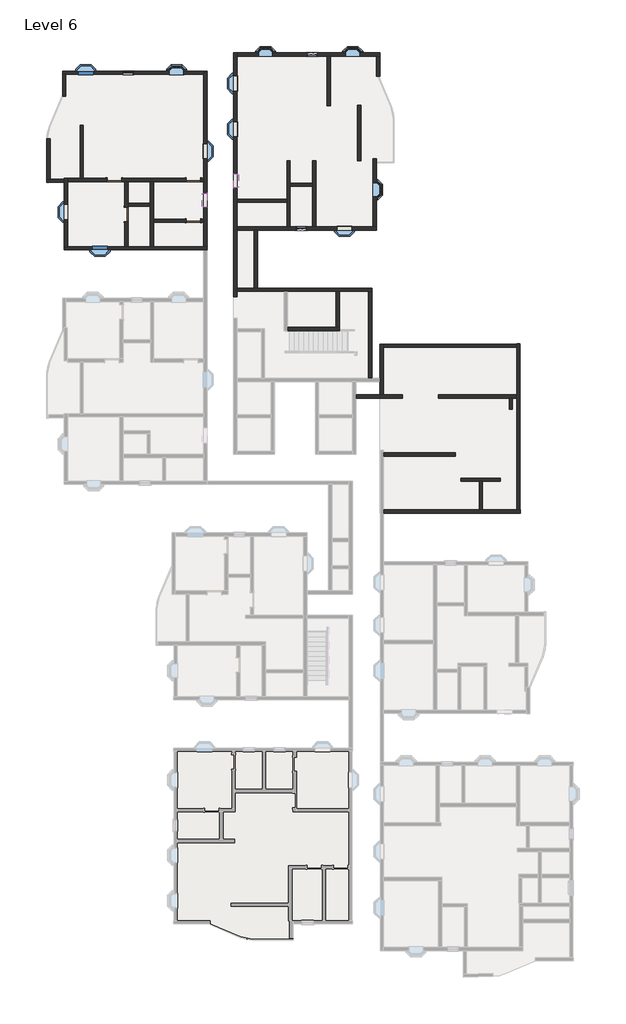
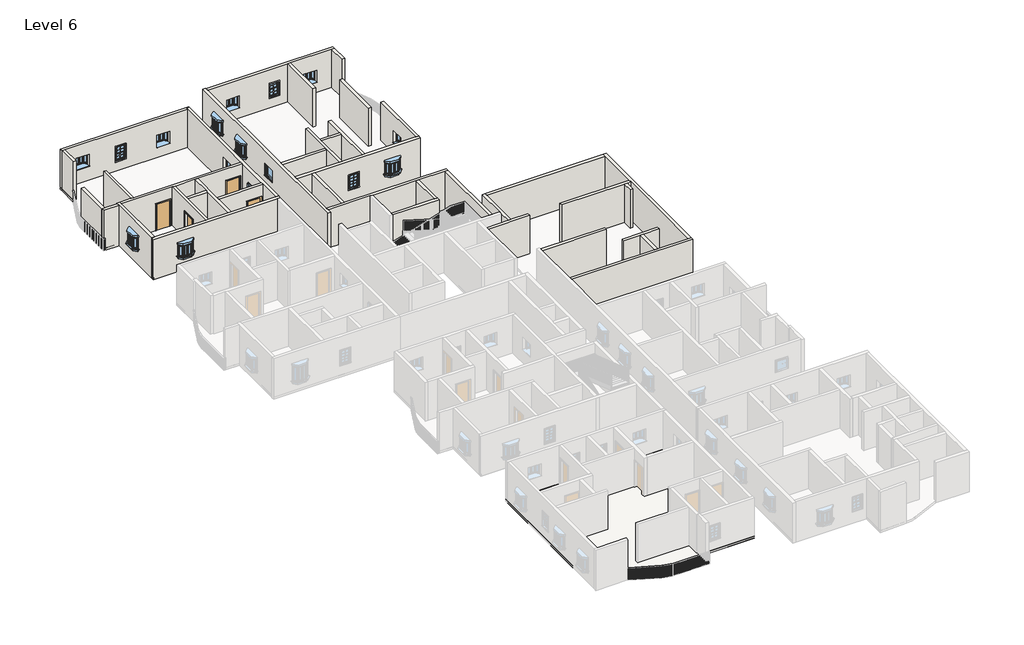
# One storey, part 4 of 14: 39 walls, 16 windows, 4 doors, 2 roofs.
"""IFC4 building model written with IfcOpenShell, lengths in millimetres."""

from ifc_helpers import new_model, si_unit, point, frame, frame_2d, origin, place, context, project, spatial, polyline, circle_curve, trimmed, segment, composite_curve, outline, extrude, faceted_brep, transform, mapped, element, save
from components import door_719f80de, window_910x910mm_67ef725a, window_8debb0fa, windows_sgl_w_glazing_bars_910x910mm_256712d0

model = new_model("IFC4")

# Units and contexts
model_context = context("Model", 3, world=origin())
ifc_project = project(units=[si_unit("LENGTHUNIT", "METRE", prefix="MILLI")], contexts=[model_context])

# Site, building, storey
site = spatial("IfcSite", under=ifc_project)
building = spatial("IfcBuilding", under=site)
storey = spatial("IfcBuildingStorey", under=building, Name="Level 6", Elevation=15240.0)

# Doors
placement = place(None, origin())
door_shape = door_719f80de(model_context)
element("IfcDoor", 1, ObjectType="Single-Flush : 36\" x 84\"", at=placement, inside=storey, context=model_context, shape_type="MappedRepresentation", body=[
    mapped(door_shape, transform((-16068.1391351, 22048.4083494, 15240.0), x_axis=(1.0, 0.0, 0.0), y_axis=(0.0, 1.0, 0.0), z_axis=(0.0, 0.0, 1.0))),
])
element("IfcDoor", 2, ObjectType="Single-Flush : 36\" x 84\"", at=placement, inside=storey, context=model_context, shape_type="MappedRepresentation", body=[
    mapped(door_shape, transform((-15306.1391351, 19864.0083494, 15240.0), x_axis=(0.0, 1.0, 0.0), y_axis=(-1.0, 0.0, 0.0), z_axis=(0.0, 0.0, 1.0))),
])
element("IfcDoor", 3, ObjectType="Single-Flush : 36\" x 84\"", at=placement, inside=storey, context=model_context, shape_type="MappedRepresentation", body=[
    mapped(door_shape, transform((-11057.9891351, 19470.3083494, 15240.0), x_axis=(1.0, 0.0, 0.0), y_axis=(0.0, 1.0, 0.0), z_axis=(0.0, 0.0, 1.0))),
])
element("IfcDoor", 4, ObjectType="Single-Flush : 36\" x 84\"", at=placement, inside=storey, context=model_context, shape_type="MappedRepresentation", body=[
    mapped(door_shape, transform((-11057.9891351, 22048.4083494, 15240.0), x_axis=(1.0, 0.0, 0.0), y_axis=(0.0, 1.0, 0.0), z_axis=(0.0, 0.0, 1.0))),
])

# Roofs
element("IfcRoof", 5, ObjectType="Generic - 12\"", at=placement, inside=storey, context=model_context, shape_type="SweptSolid", body=[
    extrude(outline(composite_curve([segment(polyline([(-10024.8708389, -25100.3416506), (-12290.487215, -25100.3416506), (-12290.487215, -13962.4416506), (-986.8891351, -13962.4416506), (-986.8891351, -25100.3416506), (-4746.0891351, -25100.3416506), (-4746.0891351, -26090.9416506), (-7315.6413127, -26090.9416506)]), True, "CONTINUOUS"), segment(trimmed(circle_curve(frame_2d((-7315.6413127, -24160.5416506)), 1930.4), [point((-7315.6413127, -26090.9416506))], [point((-8075.5356374, -25935.0851906))], False, "CARTESIAN"), True, "CONTINUOUS"), segment(polyline([(-8075.5356374, -25935.0851906), (-10024.8708389, -25100.3416506)]), True, "CONTINUOUS")], self_intersect=False)), frame((0.0, 0.0, 15240.0), z_axis=(0.0, 0.0, 1.0), x_axis=(1.0, 0.0, 0.0)), (0.0, 0.0, 1.0), 152.4),
])
element("IfcRoof", 6, ObjectType="Generic - 12\"", at=placement, inside=storey, context=model_context, shape_type="SweptSolid", body=[
    extrude(outline(composite_curve([segment(polyline([(-10024.8708389, -25100.3416506), (-12290.487215, -25100.3416506), (-12290.487215, -13962.4416506), (-986.8891351, -13962.4416506), (-986.8891351, -25100.3416506), (-4746.0891351, -25100.3416506), (-4746.0891351, -26090.9416506), (-7315.6413127, -26090.9416506)]), True, "CONTINUOUS"), segment(trimmed(circle_curve(frame_2d((-7315.6413127, -24160.5416506)), 1930.4), [point((-7315.6413127, -26090.9416506))], [point((-8075.5356374, -25935.0851906))], False, "CARTESIAN"), True, "CONTINUOUS"), segment(polyline([(-8075.5356374, -25935.0851906), (-10024.8708389, -25100.3416506)]), True, "CONTINUOUS")], self_intersect=False)), frame((0.0, 0.0, 15240.0), z_axis=(0.0, 0.0, 1.0), x_axis=(1.0, 0.0, 0.0)), (0.0, 0.0, 1.0), 152.4),
])

# Walls
element("IfcWall", 7, ObjectType="4.5\" p", at=placement, inside=storey, context=model_context, shape_type="Brep", body=[
    faceted_brep([(-10600.7891351, 21946.8083494, 17373.6), (-10600.7891351, 21946.8083494, 15240.0), (-10397.5891351, 21946.8083494, 15240.0), (-10397.5891351, 21946.8083494, 18288.0), (-13578.9391351, 21946.8083494, 18288.0), (-13782.1391351, 21946.8083494, 18288.0), (-15204.5391351, 21946.8083494, 18288.0), (-15407.7391351, 21946.8083494, 18288.0), (-19033.5891351, 21946.8083494, 18288.0), (-19033.5891351, 21946.8083494, 15240.0), (-16525.3391351, 21946.8083494, 15240.0), (-16525.3391351, 21946.8083494, 17373.6), (-15610.9391351, 21946.8083494, 17373.6), (-15610.9391351, 21946.8083494, 15240.0), (-15407.7391351, 21946.8083494, 15240.0), (-15204.5391351, 21946.8083494, 15240.0), (-13782.1391351, 21946.8083494, 15240.0), (-13578.9391351, 21946.8083494, 15240.0), (-11515.1891351, 21946.8083494, 15240.0), (-11515.1891351, 21946.8083494, 17373.6), (-10397.5891351, 22150.0083494, 15240.0), (-10600.7891351, 22150.0083494, 15240.0), (-10600.7891351, 22150.0083494, 17373.6), (-11515.1891351, 22150.0083494, 17373.6), (-11515.1891351, 22150.0083494, 15240.0), (-15610.9391351, 22150.0083494, 15240.0), (-15610.9391351, 22150.0083494, 17373.6), (-16525.3391351, 22150.0083494, 17373.6), (-16525.3391351, 22150.0083494, 15240.0), (-18042.9891351, 22150.0083494, 15240.0), (-18246.1891351, 22150.0083494, 15240.0), (-19033.5891351, 22150.0083494, 15240.0), (-19033.5891351, 22150.0083494, 18288.0), (-18246.1891351, 22150.0083494, 18288.0), (-18042.9891351, 22150.0083494, 18288.0), (-10397.5891351, 22150.0083494, 18288.0)], [[[0, 1, 2, 3, 4, 5, 6, 7, 8, 9, 10, 11, 12, 13, 14, 15, 16, 17, 18, 19]], [[20, 21, 22, 23, 24, 25, 26, 27, 28, 29, 30, 31, 32, 33, 34, 35]], [[10, 9, 31, 30, 29, 28]], [[2, 1, 21, 20]], [[18, 17, 16, 15, 14, 13, 25, 24]], [[8, 7, 6, 5, 4, 3, 35, 34, 33, 32]], [[9, 8, 32, 31]], [[3, 2, 20, 35]], [[26, 25, 13, 12]], [[27, 26, 12, 11]], [[28, 27, 11, 10]], [[22, 21, 1, 0]], [[23, 22, 0, 19]], [[24, 23, 19, 18]]]),
])
element("IfcWall", 8, ObjectType="4.5\" p", at=placement, inside=storey, context=model_context, shape_type="Brep", body=[
    faceted_brep([(-15407.7391351, 21946.8083494, 15240.0), (-15407.7391351, 20321.2083494, 15240.0), (-15407.7391351, 20321.2083494, 17373.6), (-15407.7391351, 19406.8083494, 17373.6), (-15407.7391351, 19406.8083494, 15240.0), (-15407.7391351, 17812.9583494, 15240.0), (-15407.7391351, 17812.9583494, 18288.0), (-15407.7391351, 21946.8083494, 18288.0), (-15204.5391351, 20321.2083494, 17373.6), (-15204.5391351, 20321.2083494, 15240.0), (-15204.5391351, 20372.0083494, 15240.0), (-15204.5391351, 20575.2083494, 15240.0), (-15204.5391351, 21946.8083494, 15240.0), (-15204.5391351, 21946.8083494, 18288.0), (-15204.5391351, 20575.2083494, 18288.0), (-15204.5391351, 20372.0083494, 18288.0), (-15204.5391351, 17812.9583494, 18288.0), (-15204.5391351, 17812.9583494, 15240.0), (-15204.5391351, 19406.8083494, 15240.0), (-15204.5391351, 19406.8083494, 17373.6)], [[[0, 1, 2, 3, 4, 5, 6, 7]], [[8, 9, 10, 11, 12, 13, 14, 15, 16, 17, 18, 19]], [[18, 17, 5, 4]], [[12, 11, 10, 9, 1, 0]], [[7, 6, 16, 15, 14, 13]], [[6, 5, 17, 16]], [[0, 7, 13, 12]], [[2, 1, 9, 8]], [[3, 2, 8, 19]], [[4, 3, 19, 18]]]),
])
element("IfcWall", 9, ObjectType="4.5\" p", at=placement, inside=storey, context=model_context, shape_type="Brep", body=[
    faceted_brep([(-13782.1391351, 21946.8083494, 15240.0), (-13782.1391351, 20575.2083494, 15240.0), (-13782.1391351, 20372.0083494, 15240.0), (-13782.1391351, 17812.9583494, 15240.0), (-13782.1391351, 17812.9583494, 18288.0), (-13782.1391351, 20372.0083494, 18288.0), (-13782.1391351, 20575.2083494, 18288.0), (-13782.1391351, 21946.8083494, 18288.0), (-13578.9391351, 21946.8083494, 15240.0), (-13578.9391351, 21946.8083494, 18288.0), (-13578.9391351, 19571.9083494, 18288.0), (-13578.9391351, 19368.7083494, 18288.0), (-13578.9391351, 17812.9583494, 18288.0), (-13578.9391351, 17812.9583494, 15240.0), (-13578.9391351, 19368.7083494, 15240.0), (-13578.9391351, 19571.9083494, 15240.0)], [[[0, 1, 2, 3, 4, 5, 6, 7]], [[8, 9, 10, 11, 12, 13, 14, 15]], [[3, 2, 1, 0, 8, 15, 14, 13]], [[7, 6, 5, 4, 12, 11, 10, 9]], [[4, 3, 13, 12]], [[0, 7, 9, 8]]]),
])
element("IfcWall", 10, ObjectType="4.5\" p", at=placement, inside=storey, context=model_context, shape_type="SweptSolid", body=[
    extrude(outline(polyline([(-13782.1391351, 20372.0083494), (-15204.5391351, 20372.0083494), (-15204.5391351, 20575.2083494), (-13782.1391351, 20575.2083494), (-13782.1391351, 20372.0083494)])), frame((0.0, 0.0, 15240.0), z_axis=(0.0, 0.0, 1.0), x_axis=(1.0, 0.0, 0.0)), (0.0, 0.0, 1.0), 3048.0),
])
element("IfcWall", 11, ObjectType="4.5\" p", at=placement, inside=storey, context=model_context, shape_type="SweptSolid", body=[
    extrude(outline(polyline([(17373.6, -10600.7891351), (15240.0, -10600.7891351), (15240.0, -10397.5891351), (18288.0, -10397.5891351), (18288.0, -13578.9391351), (15240.0, -13578.9391351), (15240.0, -11515.1891351), (17373.6, -11515.1891351), (17373.6, -10600.7891351)])), frame((0.0, 19368.7083494, 0.0), z_axis=(0.0, 1.0, 0.0), x_axis=(0.0, 0.0, 1.0)), (0.0, 0.0, 1.0), 203.2),
])
element("IfcWall", 12, ObjectType="4.5\" p", at=placement, inside=storey, context=model_context, shape_type="SweptSolid", body=[
    extrude(outline(polyline([(-18246.1891351, 22150.0083494), (-18246.1891351, 25515.5083494), (-18042.9891351, 25515.5083494), (-18042.9891351, 22150.0083494), (-18246.1891351, 22150.0083494)])), frame((0.0, 0.0, 15240.0), z_axis=(0.0, 0.0, 1.0), x_axis=(1.0, 0.0, 0.0)), (0.0, 0.0, 1.0), 3048.0),
])
element("IfcWall", 13, ObjectType="4.5\" p", at=placement, inside=storey, context=model_context, shape_type="SweptSolid", body=[
    extrude(outline(polyline([(-6993.9891351, 18875.1215905), (-6993.9891351, 15192.1215905), (-7197.1891351, 15192.1215905), (-7197.1891351, 18875.1215905), (-6993.9891351, 18875.1215905)])), frame((0.0, 0.0, 15240.0), z_axis=(0.0, 0.0, 1.0), x_axis=(1.0, 0.0, 0.0)), (0.0, 0.0, 1.0), 3048.0),
])
element("IfcWall", 14, ObjectType="4.5\" p", at=placement, inside=storey, context=model_context, shape_type="Brep", body=[
    faceted_brep([(-8289.3891351, 18875.1215905, 15240.0), (-7197.1891351, 18875.1215905, 15240.0), (-6993.9891351, 18875.1215905, 15240.0), (562.5108649, 18875.1215905, 15240.0), (562.5108649, 18875.1215905, 18288.0), (-6993.9891351, 18875.1215905, 18288.0), (-7197.1891351, 18875.1215905, 18288.0), (-8289.3891351, 18875.1215905, 18288.0), (-1017.6641351, 18875.1215905, 17350.0), (-1017.6641351, 18875.1215905, 16440.0), (-1927.6641351, 18875.1215905, 16440.0), (-1927.6641351, 18875.1215905, 17350.0), (-3876.1391351, 18875.1215905, 17221.2), (-3876.1391351, 18875.1215905, 16154.4), (-4536.5391351, 18875.1215905, 16154.4), (-4536.5391351, 18875.1215905, 17221.2), (-8289.3891351, 19078.3215905, 15240.0), (-8289.3891351, 19078.3215905, 18288.0), (-5120.7391351, 19078.3215905, 18288.0), (-4917.5391351, 19078.3215905, 18288.0), (-3495.1391351, 19078.3215905, 18288.0), (-3291.9391351, 19078.3215905, 18288.0), (346.6108649, 19078.3215905, 18288.0), (549.8108649, 19078.3215905, 18288.0), (562.5108649, 19078.3215905, 18288.0), (562.5108649, 19078.3215905, 15240.0), (549.8108649, 19078.3215905, 15240.0), (346.6108649, 19078.3215905, 15240.0), (-3291.9391351, 19078.3215905, 15240.0), (-3495.1391351, 19078.3215905, 15240.0), (-4917.5391351, 19078.3215905, 15240.0), (-5120.7391351, 19078.3215905, 15240.0), (-1017.6641351, 19078.3215905, 17350.0), (-1927.6641351, 19078.3215905, 17350.0), (-1927.6641351, 19078.3215905, 16440.0), (-1017.6641351, 19078.3215905, 16440.0), (-3876.1391351, 19078.3215905, 17221.2), (-4536.5391351, 19078.3215905, 17221.2), (-4536.5391351, 19078.3215905, 16154.4), (-3876.1391351, 19078.3215905, 16154.4)], [[[0, 1, 2, 3, 4, 5, 6, 7], [8, 9, 10, 11], [12, 13, 14, 15]], [[16, 17, 18, 19, 20, 21, 22, 23, 24, 25, 26, 27, 28, 29, 30, 31], [32, 33, 34, 35], [36, 37, 38, 39]], [[3, 2, 1, 0, 16, 31, 30, 29, 28, 27, 26, 25]], [[4, 3, 25, 24]], [[7, 6, 5, 4, 24, 23, 22, 21, 20, 19, 18, 17]], [[0, 7, 17, 16]], [[9, 8, 32, 35]], [[10, 9, 35, 34]], [[11, 10, 34, 33]], [[8, 11, 33, 32]], [[13, 12, 36, 39]], [[14, 13, 39, 38]], [[15, 14, 38, 37]], [[12, 15, 37, 36]]]),
])
element("IfcWall", 15, ObjectType="4.5\" p", at=placement, inside=storey, context=model_context, shape_type="SweptSolid", body=[
    extrude(outline(polyline([(19078.3215905, 15240.0), (19078.3215905, 18288.0), (23396.3215905, 18288.0), (23396.3215905, 15240.0), (19078.3215905, 15240.0)]), holes=[polyline([(21882.8215905, 17064.4), (20972.8215905, 17064.4), (20972.8215905, 16154.4), (21882.8215905, 16154.4), (21882.8215905, 17064.4)])]), frame((346.6108649, 0.0, 0.0), z_axis=(1.0, 0.0, 0.0), x_axis=(0.0, 1.0, 0.0)), (0.0, 0.0, 1.0), 203.2),
])
element("IfcWall", 16, ObjectType="4.5\" p", at=placement, inside=storey, context=model_context, shape_type="SweptSolid", body=[
    extrude(outline(polyline([(-5120.7391351, 20634.0715905), (-8289.3891351, 20634.0715905), (-8289.3891351, 20837.2715905), (-5120.7391351, 20837.2715905), (-5120.7391351, 20634.0715905)])), frame((0.0, 0.0, 15240.0), z_axis=(0.0, 0.0, 1.0), x_axis=(1.0, 0.0, 0.0)), (0.0, 0.0, 1.0), 3048.0),
])
element("IfcWall", 17, ObjectType="4.5\" p", at=placement, inside=storey, context=model_context, shape_type="Brep", body=[
    faceted_brep([(-5120.7391351, 23256.6215905, 15240.0), (-5120.7391351, 20837.2715905, 15240.0), (-5120.7391351, 20634.0715905, 15240.0), (-5120.7391351, 19078.3215905, 15240.0), (-5120.7391351, 19078.3215905, 18288.0), (-5120.7391351, 20634.0715905, 18288.0), (-5120.7391351, 20837.2715905, 18288.0), (-5120.7391351, 23256.6215905, 18288.0), (-4917.5391351, 23256.6215905, 15240.0), (-4917.5391351, 23256.6215905, 18288.0), (-4917.5391351, 21853.2715905, 18288.0), (-4917.5391351, 21650.0715905, 18288.0), (-4917.5391351, 19078.3215905, 18288.0), (-4917.5391351, 19078.3215905, 15240.0), (-4917.5391351, 21650.0715905, 15240.0), (-4917.5391351, 21853.2715905, 15240.0)], [[[0, 1, 2, 3, 4, 5, 6, 7]], [[8, 9, 10, 11, 12, 13, 14, 15]], [[3, 2, 1, 0, 8, 15, 14, 13]], [[7, 6, 5, 4, 12, 11, 10, 9]], [[0, 7, 9, 8]], [[4, 3, 13, 12]]]),
])
element("IfcWall", 18, ObjectType="4.5\" p", at=placement, inside=storey, context=model_context, shape_type="Brep", body=[
    faceted_brep([(-3495.1391351, 23256.6215905, 15240.0), (-3495.1391351, 21853.2715905, 15240.0), (-3495.1391351, 21650.0715905, 15240.0), (-3495.1391351, 19078.3215905, 15240.0), (-3495.1391351, 19078.3215905, 18288.0), (-3495.1391351, 21650.0715905, 18288.0), (-3495.1391351, 21853.2715905, 18288.0), (-3495.1391351, 23256.6215905, 18288.0), (-3291.9391351, 23256.6215905, 15240.0), (-3291.9391351, 23256.6215905, 18288.0), (-3291.9391351, 19078.3215905, 18288.0), (-3291.9391351, 19078.3215905, 15240.0)], [[[0, 1, 2, 3, 4, 5, 6, 7]], [[8, 9, 10, 11]], [[3, 2, 1, 0, 8, 11]], [[7, 6, 5, 4, 10, 9]], [[0, 7, 9, 8]], [[4, 3, 11, 10]]]),
])
element("IfcWall", 19, ObjectType="4.5\" p", at=placement, inside=storey, context=model_context, shape_type="SweptSolid", body=[
    extrude(outline(polyline([(-3495.1391351, 21650.0715905), (-4917.5391351, 21650.0715905), (-4917.5391351, 21853.2715905), (-3495.1391351, 21853.2715905), (-3495.1391351, 21650.0715905)])), frame((0.0, 0.0, 15240.0), z_axis=(0.0, 0.0, 1.0), x_axis=(1.0, 0.0, 0.0)), (0.0, 0.0, 1.0), 3048.0),
])
element("IfcWall", 20, ObjectType="4.5\" p", at=placement, inside=storey, context=model_context, shape_type="SweptSolid", body=[
    extrude(outline(polyline([(-1799.6891351, 14988.9215905), (-1799.6891351, 12709.2715905), (-2002.8891351, 12709.2715905), (-2002.8891351, 14988.9215905), (-1799.6891351, 14988.9215905)])), frame((0.0, 0.0, 15240.0), z_axis=(0.0, 0.0, 1.0), x_axis=(1.0, 0.0, 0.0)), (0.0, 0.0, 1.0), 3048.0),
])
element("IfcWall", 21, ObjectType="4.5\" p", at=placement, inside=storey, context=model_context, shape_type="Brep", body=[
    faceted_brep([(-5095.3391351, 12506.0715905, 15240.0), (-1786.9891351, 12506.0715905, 15240.0), (-1786.9891351, 12506.0715905, 18288.0), (-5095.3391351, 12506.0715905, 18288.0), (-5095.3391351, 12709.2715905, 15240.0), (-5095.3391351, 12709.2715905, 18288.0), (-2002.8891351, 12709.2715905, 18288.0), (-1799.6891351, 12709.2715905, 18288.0), (-1786.9891351, 12709.2715905, 18288.0), (-1786.9891351, 12709.2715905, 15240.0), (-1799.6891351, 12709.2715905, 15240.0), (-2002.8891351, 12709.2715905, 15240.0)], [[[0, 1, 2, 3]], [[4, 5, 6, 7, 8, 9, 10, 11]], [[1, 0, 4, 11, 10, 9]], [[2, 1, 9, 8]], [[3, 2, 8, 7, 6, 5]], [[0, 3, 5, 4]]]),
])
element("IfcWall", 22, ObjectType="4.5\" p", at=placement, inside=storey, context=model_context, shape_type="Brep", body=[
    faceted_brep([(-745.5891351, 8223.6457306, 15240.0), (2209.4205024, 8223.6457306, 15240.0), (2209.4205024, 8223.6457306, 18288.0), (-745.5891351, 8223.6457306, 18288.0), (-745.5891351, 8426.8457306, 15240.0), (-745.5891351, 8426.8457306, 18288.0), (793.5880523, 8426.8457306, 18288.0), (996.7880523, 8426.8457306, 18288.0), (2209.4205024, 8426.8457306, 18288.0), (2209.4205024, 8426.8457306, 15240.0), (996.7880523, 8426.8457306, 15240.0), (793.5880523, 8426.8457306, 15240.0)], [[[0, 1, 2, 3]], [[4, 5, 6, 7, 8, 9, 10, 11]], [[1, 0, 4, 11, 10, 9]], [[2, 1, 9, 8]], [[3, 2, 8, 7, 6, 5]], [[0, 3, 5, 4]]]),
])
element("IfcWall", 23, ObjectType="4.5\" p", at=placement, inside=storey, context=model_context, shape_type="Brep", body=[
    faceted_brep([(996.7880523, 8426.8457306, 15240.0), (996.7880523, 11443.0957306, 15240.0), (996.7880523, 11646.2957306, 15240.0), (996.7880523, 11646.2957306, 18288.0), (996.7880523, 11443.0957306, 18288.0), (996.7880523, 8426.8457306, 18288.0), (793.5880523, 8426.8457306, 15240.0), (793.5880523, 8426.8457306, 18288.0), (793.5880523, 9275.2949943, 18288.0), (793.5880523, 9478.4949943, 18288.0), (793.5880523, 11646.2957306, 18288.0), (793.5880523, 11646.2957306, 15240.0), (793.5880523, 9478.4949943, 15240.0), (793.5880523, 9275.2949943, 15240.0)], [[[0, 1, 2, 3, 4, 5]], [[6, 7, 8, 9, 10, 11, 12, 13]], [[2, 1, 0, 6, 13, 12, 11]], [[5, 4, 3, 10, 9, 8, 7]], [[0, 5, 7, 6]], [[3, 2, 11, 10]]]),
])
element("IfcWall", 24, ObjectType="4.5\" p", at=placement, inside=storey, context=model_context, shape_type="Brep", body=[
    faceted_brep([(9461.3380523, 8426.8457306, 15240.0), (4492.3034266, 8426.8457306, 15240.0), (4492.3034266, 8426.8457306, 18288.0), (9461.3380523, 8426.8457306, 18288.0), (9461.3380523, 8223.6457306, 15240.0), (9461.3380523, 8223.6457306, 18288.0), (9181.9380523, 8223.6457306, 18288.0), (8978.7380523, 8223.6457306, 18288.0), (4492.3034266, 8223.6457306, 18288.0), (4492.3034266, 8223.6457306, 15240.0), (8978.7380523, 8223.6457306, 15240.0), (9181.9380523, 8223.6457306, 15240.0)], [[[0, 1, 2, 3]], [[4, 5, 6, 7, 8, 9, 10, 11]], [[1, 0, 4, 11, 10, 9]], [[2, 1, 9, 8]], [[3, 2, 8, 7, 6, 5]], [[0, 3, 5, 4]]]),
])
element("IfcWall", 25, ObjectType="4.5\" p", at=placement, inside=storey, context=model_context, shape_type="Brep", body=[
    faceted_brep([(1007.0108649, 940.1957306, 15240.0), (9677.2380523, 940.1957306, 15240.0), (9677.2380523, 940.1957306, 18288.0), (1007.0108649, 940.1957306, 18288.0), (1007.0108649, 1143.3957306, 15240.0), (1007.0108649, 1143.3957306, 18288.0), (7073.7380523, 1143.3957306, 18288.0), (7276.9380523, 1143.3957306, 18288.0), (9461.3380523, 1143.3957306, 18288.0), (9664.5380523, 1143.3957306, 18288.0), (9677.2380523, 1143.3957306, 18288.0), (9677.2380523, 1143.3957306, 15240.0), (9664.5380523, 1143.3957306, 15240.0), (9461.3380523, 1143.3957306, 15240.0), (7276.9380523, 1143.3957306, 15240.0), (7073.7380523, 1143.3957306, 15240.0)], [[[0, 1, 2, 3]], [[4, 5, 6, 7, 8, 9, 10, 11, 12, 13, 14, 15]], [[1, 0, 4, 15, 14, 13, 12, 11]], [[2, 1, 11, 10]], [[3, 2, 10, 9, 8, 7, 6, 5]], [[0, 3, 5, 4]]]),
])
element("IfcWall", 26, ObjectType="4.5\" p", at=placement, inside=storey, context=model_context, shape_type="Brep", body=[
    faceted_brep([(9664.5380523, 1143.3957306, 15240.0), (9664.5380523, 11658.9957306, 15240.0), (9664.5380523, 11658.9957306, 18288.0), (9664.5380523, 1143.3957306, 18288.0), (9461.3380523, 1143.3957306, 15240.0), (9461.3380523, 1143.3957306, 18288.0), (9461.3380523, 8223.6457306, 18288.0), (9461.3380523, 8426.8457306, 18288.0), (9461.3380523, 11443.0957306, 18288.0), (9461.3380523, 11646.2957306, 18288.0), (9461.3380523, 11658.9957306, 18288.0), (9461.3380523, 11658.9957306, 15240.0), (9461.3380523, 11646.2957306, 15240.0), (9461.3380523, 11443.0957306, 15240.0), (9461.3380523, 8426.8457306, 15240.0), (9461.3380523, 8223.6457306, 15240.0)], [[[0, 1, 2, 3]], [[4, 5, 6, 7, 8, 9, 10, 11, 12, 13, 14, 15]], [[1, 0, 4, 15, 14, 13, 12, 11]], [[2, 1, 11, 10]], [[3, 2, 10, 9, 8, 7, 6, 5]], [[0, 3, 5, 4]]]),
])
element("IfcWall", 27, ObjectType="4.5\" p", at=placement, inside=storey, context=model_context, shape_type="SweptSolid", body=[
    extrude(outline(polyline([(-643.9891351, 23256.6215905), (-643.9891351, 26780.8715905), (-440.7891351, 26780.8715905), (-440.7891351, 23256.6215905), (-643.9891351, 23256.6215905)])), frame((0.0, 0.0, 15240.0), z_axis=(0.0, 0.0, 1.0), x_axis=(1.0, 0.0, 0.0)), (0.0, 0.0, 1.0), 3048.0),
])
element("IfcWall", 28, ObjectType="4.5\" p", at=placement, inside=storey, context=model_context, shape_type="SweptSolid", body=[
    extrude(outline(polyline([(-2568.0391351, 26760.9286213), (-2568.0391351, 29898.7215905), (-2364.8391351, 29898.7215905), (-2364.8391351, 26760.9286213), (-2568.0391351, 26760.9286213)])), frame((0.0, 0.0, 15240.0), z_axis=(0.0, 0.0, 1.0), x_axis=(1.0, 0.0, 0.0)), (0.0, 0.0, 1.0), 3048.0),
])
element("IfcWall", 29, ObjectType="4.5\" p", at=placement, inside=storey, context=model_context, shape_type="SweptSolid", body=[
    extrude(outline(polyline([(765.7108649, 29898.7215905), (765.7108649, 28631.1875845), (562.5108649, 28631.1875845), (562.5108649, 29898.7215905), (765.7108649, 29898.7215905)])), frame((0.0, 0.0, 15240.0), z_axis=(0.0, 0.0, 1.0), x_axis=(1.0, 0.0, 0.0)), (0.0, 0.0, 1.0), 3048.0),
])
element("IfcWall", 30, ObjectType="9\" w", at=placement, inside=storey, context=model_context, shape_type="Brep", body=[
    faceted_brep([(-10181.6891351, 17812.9583494, 15240.0), (-10194.3891351, 17812.9583494, 15240.0), (-10397.5891351, 17812.9583494, 15240.0), (-13578.9391351, 17812.9583494, 15240.0), (-13782.1391351, 17812.9583494, 15240.0), (-15204.5391351, 17812.9583494, 15240.0), (-15407.7391351, 17812.9583494, 15240.0), (-19033.5891351, 17812.9583494, 15240.0), (-19236.7891351, 17812.9583494, 15240.0), (-19249.4891351, 17812.9583494, 15240.0), (-19249.4891351, 17812.9583494, 18288.0), (-19236.7891351, 17812.9583494, 18288.0), (-19033.5891351, 17812.9583494, 18288.0), (-15407.7391351, 17812.9583494, 18288.0), (-15204.5391351, 17812.9583494, 18288.0), (-13782.1391351, 17812.9583494, 18288.0), (-13578.9391351, 17812.9583494, 18288.0), (-10397.5891351, 17812.9583494, 18288.0), (-10194.3891351, 17812.9583494, 18288.0), (-10181.6891351, 17812.9583494, 18288.0), (-16527.5391351, 17812.9583494, 17350.0), (-17437.5391351, 17812.9583494, 17350.0), (-17437.5391351, 17812.9583494, 16440.0), (-16527.5391351, 17812.9583494, 16440.0), (-10181.6891351, 17609.7583494, 15240.0), (-10181.6891351, 17609.7583494, 18288.0), (-19249.4891351, 17609.7583494, 18288.0), (-19249.4891351, 17609.7583494, 15240.0), (-16527.5391351, 17609.7583494, 17350.0), (-16527.5391351, 17609.7583494, 16440.0), (-17437.5391351, 17609.7583494, 16440.0), (-17437.5391351, 17609.7583494, 17350.0)], [[[0, 1, 2, 3, 4, 5, 6, 7, 8, 9, 10, 11, 12, 13, 14, 15, 16, 17, 18, 19], [20, 21, 22, 23]], [[24, 25, 26, 27], [28, 29, 30, 31]], [[9, 8, 7, 6, 5, 4, 3, 2, 1, 0, 24, 27]], [[10, 9, 27, 26]], [[19, 18, 17, 16, 15, 14, 13, 12, 11, 10, 26, 25]], [[0, 19, 25, 24]], [[29, 28, 20, 23]], [[30, 29, 23, 22]], [[31, 30, 22, 21]], [[28, 31, 21, 20]]]),
])
element("IfcWall", 31, ObjectType="9\" w", at=placement, inside=storey, context=model_context, shape_type="Brep", body=[
    faceted_brep([(-19033.5891351, 17812.9583494, 15240.0), (-19033.5891351, 21946.8083494, 15240.0), (-19033.5891351, 22150.0083494, 15240.0), (-19033.5891351, 22150.0083494, 18288.0), (-19033.5891351, 21946.8083494, 18288.0), (-19033.5891351, 17812.9583494, 18288.0), (-19033.5891351, 19555.0583494, 17350.0), (-19033.5891351, 20465.0583494, 17350.0), (-19033.5891351, 20465.0583494, 16440.0), (-19033.5891351, 19555.0583494, 16440.0), (-19236.7891351, 17812.9583494, 15240.0), (-19236.7891351, 17812.9583494, 18288.0), (-19236.7891351, 21889.6583494, 18288.0), (-19236.7891351, 22092.8583494, 18288.0), (-19236.7891351, 22150.0083494, 18288.0), (-19236.7891351, 22150.0083494, 15240.0), (-19236.7891351, 22092.8583494, 15240.0), (-19236.7891351, 21889.6583494, 15240.0), (-19236.7891351, 19555.0583494, 17350.0), (-19236.7891351, 19555.0583494, 16440.0), (-19236.7891351, 20465.0583494, 16440.0), (-19236.7891351, 20465.0583494, 17350.0)], [[[0, 1, 2, 3, 4, 5], [6, 7, 8, 9]], [[10, 11, 12, 13, 14, 15, 16, 17], [18, 19, 20, 21]], [[2, 1, 0, 10, 17, 16, 15]], [[5, 4, 3, 14, 13, 12, 11]], [[0, 5, 11, 10]], [[3, 2, 15, 14]], [[19, 18, 6, 9]], [[20, 19, 9, 8]], [[21, 20, 8, 7]], [[18, 21, 7, 6]]]),
])
element("IfcWall", 32, ObjectType="9\" w", at=placement, inside=storey, context=model_context, shape_type="Brep", body=[
    faceted_brep([(-10194.3891351, 17812.9583494, 15240.0), (-10194.3891351, 28849.2583494, 15240.0), (-10194.3891351, 28849.2583494, 18288.0), (-10194.3891351, 17812.9583494, 18288.0), (-10194.3891351, 24319.5083494, 17350.0), (-10194.3891351, 24319.5083494, 16440.0), (-10194.3891351, 23409.5083494, 16440.0), (-10194.3891351, 23409.5083494, 17350.0), (-10194.3891351, 20304.3583494, 17350.0), (-10194.3891351, 21214.3583494, 17350.0), (-10194.3891351, 21214.3583494, 16440.0), (-10194.3891351, 20304.3583494, 16440.0), (-10397.5891351, 17812.9583494, 15240.0), (-10397.5891351, 17812.9583494, 18288.0), (-10397.5891351, 19368.7083494, 18288.0), (-10397.5891351, 19571.9083494, 18288.0), (-10397.5891351, 21946.8083494, 18288.0), (-10397.5891351, 22150.0083494, 18288.0), (-10397.5891351, 28849.2583494, 18288.0), (-10397.5891351, 28849.2583494, 15240.0), (-10397.5891351, 22150.0083494, 15240.0), (-10397.5891351, 21946.8083494, 15240.0), (-10397.5891351, 19571.9083494, 15240.0), (-10397.5891351, 19368.7083494, 15240.0), (-10397.5891351, 24319.5083494, 17350.0), (-10397.5891351, 23409.5083494, 17350.0), (-10397.5891351, 23409.5083494, 16440.0), (-10397.5891351, 24319.5083494, 16440.0), (-10397.5891351, 20304.3583494, 17350.0), (-10397.5891351, 20304.3583494, 16440.0), (-10397.5891351, 21214.3583494, 16440.0), (-10397.5891351, 21214.3583494, 17350.0)], [[[0, 1, 2, 3], [4, 5, 6, 7], [8, 9, 10, 11]], [[12, 13, 14, 15, 16, 17, 18, 19, 20, 21, 22, 23], [24, 25, 26, 27], [28, 29, 30, 31]], [[1, 0, 12, 23, 22, 21, 20, 19]], [[2, 1, 19, 18]], [[3, 2, 18, 17, 16, 15, 14, 13]], [[0, 3, 13, 12]], [[5, 4, 24, 27]], [[6, 5, 27, 26]], [[7, 6, 26, 25]], [[4, 7, 25, 24]], [[29, 28, 8, 11]], [[30, 29, 11, 10]], [[31, 30, 10, 9]], [[28, 31, 9, 8]]]),
])
element("IfcWall", 33, ObjectType="9\" w", at=placement, inside=storey, context=model_context, shape_type="Brep", body=[
    faceted_brep([(-20341.6891351, 21889.6583494, 15240.0), (-19236.7891351, 21889.6583494, 15240.0), (-19236.7891351, 21889.6583494, 18288.0), (-20341.6891351, 21889.6583494, 18288.0), (-20341.6891351, 22092.8583494, 15240.0), (-20341.6891351, 22092.8583494, 18288.0), (-20138.4891351, 22092.8583494, 18288.0), (-19236.7891351, 22092.8583494, 18288.0), (-19236.7891351, 22092.8583494, 15240.0), (-20138.4891351, 22092.8583494, 15240.0)], [[[0, 1, 2, 3]], [[4, 5, 6, 7, 8, 9]], [[1, 0, 4, 9, 8]], [[3, 2, 7, 6, 5]], [[0, 3, 5, 4]], [[2, 1, 8, 7]]]),
])
element("IfcWall", 34, ObjectType="9\" w", at=placement, inside=storey, context=model_context, shape_type="SweptSolid", body=[
    extrude(outline(polyline([(-20341.6891351, 22092.8583494), (-20341.6891351, 24656.5948172), (-20138.4891351, 24656.5948172), (-20138.4891351, 22092.8583494), (-20341.6891351, 22092.8583494)])), frame((0.0, 0.0, 15240.0), z_axis=(0.0, 0.0, 1.0), x_axis=(1.0, 0.0, 0.0)), (0.0, 0.0, 1.0), 3048.0),
])
element("IfcWall", 35, ObjectType="9\" w", at=placement, inside=storey, context=model_context, shape_type="Brep", body=[
    faceted_brep([(-8492.5891351, 30114.6215905, 15240.0), (-8492.5891351, 14654.9471999, 15240.0), (-8492.5891351, 14654.9471999, 18288.0), (-8492.5891351, 30114.6215905, 18288.0), (-8492.5891351, 27703.9922564, 17350.0), (-8492.5891351, 27703.9922564, 16440.0), (-8492.5891351, 28613.9922564, 16440.0), (-8492.5891351, 28613.9922564, 17350.0), (-8492.5891351, 24808.3922564, 17350.0), (-8492.5891351, 24808.3922564, 16440.0), (-8492.5891351, 25718.3922564, 16440.0), (-8492.5891351, 25718.3922564, 17350.0), (-8492.5891351, 22451.1465905, 17350.0), (-8492.5891351, 21541.1465905, 17350.0), (-8492.5891351, 21541.1465905, 16440.0), (-8492.5891351, 22451.1465905, 16440.0), (-8289.3891351, 30114.6215905, 15240.0), (-8289.3891351, 30114.6215905, 18288.0), (-8289.3891351, 30101.9215905, 18288.0), (-8289.3891351, 29898.7215905, 18288.0), (-8289.3891351, 20837.2715905, 18288.0), (-8289.3891351, 20634.0715905, 18288.0), (-8289.3891351, 19078.3215905, 18288.0), (-8289.3891351, 18875.1215905, 18288.0), (-8289.3891351, 15192.1215905, 18288.0), (-8289.3891351, 14988.9215905, 18288.0), (-8289.3891351, 14654.9471999, 18288.0), (-8289.3891351, 14654.9471999, 15240.0), (-8289.3891351, 14988.9215905, 15240.0), (-8289.3891351, 15192.1215905, 15240.0), (-8289.3891351, 18875.1215905, 15240.0), (-8289.3891351, 19078.3215905, 15240.0), (-8289.3891351, 20634.0715905, 15240.0), (-8289.3891351, 20837.2715905, 15240.0), (-8289.3891351, 29898.7215905, 15240.0), (-8289.3891351, 30101.9215905, 15240.0), (-8289.3891351, 27703.9922564, 17350.0), (-8289.3891351, 28613.9922564, 17350.0), (-8289.3891351, 28613.9922564, 16440.0), (-8289.3891351, 27703.9922564, 16440.0), (-8289.3891351, 24808.3922564, 17350.0), (-8289.3891351, 25718.3922564, 17350.0), (-8289.3891351, 25718.3922564, 16440.0), (-8289.3891351, 24808.3922564, 16440.0), (-8289.3891351, 22451.1465905, 17350.0), (-8289.3891351, 22451.1465905, 16440.0), (-8289.3891351, 21541.1465905, 16440.0), (-8289.3891351, 21541.1465905, 17350.0)], [[[0, 1, 2, 3], [4, 5, 6, 7], [8, 9, 10, 11], [12, 13, 14, 15]], [[16, 17, 18, 19, 20, 21, 22, 23, 24, 25, 26, 27, 28, 29, 30, 31, 32, 33, 34, 35], [36, 37, 38, 39], [40, 41, 42, 43], [44, 45, 46, 47]], [[1, 0, 16, 35, 34, 33, 32, 31, 30, 29, 28, 27]], [[2, 1, 27, 26]], [[3, 2, 26, 25, 24, 23, 22, 21, 20, 19, 18, 17]], [[0, 3, 17, 16]], [[5, 4, 36, 39]], [[6, 5, 39, 38]], [[7, 6, 38, 37]], [[4, 7, 37, 36]], [[9, 8, 40, 43]], [[10, 9, 43, 42]], [[11, 10, 42, 41]], [[8, 11, 41, 40]], [[45, 44, 12, 15]], [[46, 45, 15, 14]], [[47, 46, 14, 13]], [[44, 47, 13, 12]]]),
])
element("IfcWall", 36, ObjectType="9\" w", at=placement, inside=storey, context=model_context, shape_type="Brep", body=[
    faceted_brep([(-8289.3891351, 14988.9215905, 15240.0), (-5298.5391351, 14988.9215905, 15240.0), (-5095.3391351, 14988.9215905, 15240.0), (-2002.8891351, 14988.9215905, 15240.0), (-1799.6891351, 14988.9215905, 15240.0), (54.5108649, 14988.9215905, 15240.0), (257.7108649, 14988.9215905, 15240.0), (270.4108649, 14988.9215905, 15240.0), (270.4108649, 14988.9215905, 18288.0), (257.7108649, 14988.9215905, 18288.0), (54.5108649, 14988.9215905, 18288.0), (-1799.6891351, 14988.9215905, 18288.0), (-2002.8891351, 14988.9215905, 18288.0), (-5095.3391351, 14988.9215905, 18288.0), (-5298.5391351, 14988.9215905, 18288.0), (-8289.3891351, 14988.9215905, 18288.0), (-8289.3891351, 15192.1215905, 15240.0), (-8289.3891351, 15192.1215905, 18288.0), (-7197.1891351, 15192.1215905, 18288.0), (-6993.9891351, 15192.1215905, 18288.0), (270.4108649, 15192.1215905, 18288.0), (270.4108649, 15192.1215905, 15240.0), (-6993.9891351, 15192.1215905, 15240.0), (-7197.1891351, 15192.1215905, 15240.0)], [[[0, 1, 2, 3, 4, 5, 6, 7, 8, 9, 10, 11, 12, 13, 14, 15]], [[16, 17, 18, 19, 20, 21, 22, 23]], [[7, 6, 5, 4, 3, 2, 1, 0, 16, 23, 22, 21]], [[8, 7, 21, 20]], [[15, 14, 13, 12, 11, 10, 9, 8, 20, 19, 18, 17]], [[0, 15, 17, 16]]]),
])
element("IfcWall", 37, ObjectType="9\" w", at=placement, inside=storey, context=model_context, shape_type="SweptSolid", body=[
    extrude(outline(polyline([(54.5108649, 9478.4949943), (54.5108649, 14988.9215905), (257.7108649, 14988.9215905), (257.7108649, 9478.4949943), (54.5108649, 9478.4949943)])), frame((0.0, 0.0, 15240.0), z_axis=(0.0, 0.0, 1.0), x_axis=(1.0, 0.0, 0.0)), (0.0, 0.0, 1.0), 3048.0),
])
element("IfcWall", 38, ObjectType="9\" w", at=placement, inside=storey, context=model_context, shape_type="SweptSolid", body=[
    extrude(outline(polyline([(9461.3380523, 11443.0957306), (996.7880523, 11443.0957306), (996.7880523, 11646.2957306), (9461.3380523, 11646.2957306), (9461.3380523, 11443.0957306)])), frame((0.0, 0.0, 15240.0), z_axis=(0.0, 0.0, 1.0), x_axis=(1.0, 0.0, 0.0)), (0.0, 0.0, 1.0), 3048.0),
])
element("IfcWall", 39, ObjectType="9\" w", at=placement, inside=storey, context=model_context, shape_type="SweptSolid", body=[
    extrude(outline(polyline([(8978.7380523, 7506.0957306), (8978.7380523, 8223.6457306), (9181.9380523, 8223.6457306), (9181.9380523, 7506.0957306), (8978.7380523, 7506.0957306)])), frame((0.0, 0.0, 15240.0), z_axis=(0.0, 0.0, 1.0), x_axis=(1.0, 0.0, 0.0)), (0.0, 0.0, 1.0), 3048.0),
])
element("IfcWall", 40, ObjectType="9\" w", at=placement, inside=storey, context=model_context, shape_type="SweptSolid", body=[
    extrude(outline(polyline([(7276.9380523, 2954.8622042), (7276.9380523, 1143.3957306), (7073.7380523, 1143.3957306), (7073.7380523, 2954.8622042), (7276.9380523, 2954.8622042)])), frame((0.0, 0.0, 15240.0), z_axis=(0.0, 0.0, 1.0), x_axis=(1.0, 0.0, 0.0)), (0.0, 0.0, 1.0), 3048.0),
])
element("IfcWall", 41, ObjectType="9\" w", at=placement, inside=storey, context=model_context, shape_type="Brep", body=[
    faceted_brep([(5904.1857655, 2954.8622042, 15240.0), (7073.7380523, 2954.8622042, 15240.0), (7276.9380523, 2954.8622042, 15240.0), (8418.7857655, 2954.8622042, 15240.0), (8418.7857655, 2954.8622042, 18288.0), (7276.9380523, 2954.8622042, 18288.0), (7073.7380523, 2954.8622042, 18288.0), (5904.1857655, 2954.8622042, 18288.0), (5904.1857655, 3158.0622042, 15240.0), (5904.1857655, 3158.0622042, 18288.0), (8418.7857655, 3158.0622042, 18288.0), (8418.7857655, 3158.0622042, 15240.0)], [[[0, 1, 2, 3, 4, 5, 6, 7]], [[8, 9, 10, 11]], [[3, 2, 1, 0, 8, 11]], [[4, 3, 11, 10]], [[7, 6, 5, 4, 10, 9]], [[0, 7, 9, 8]]]),
])
element("IfcWall", 42, ObjectType="9\" w", at=placement, inside=storey, context=model_context, shape_type="SweptSolid", body=[
    extrude(outline(polyline([(5571.3060189, 4550.8949943), (1007.0108649, 4550.8949943), (1007.0108649, 4754.0949943), (5571.3060189, 4754.0949943), (5571.3060189, 4550.8949943)])), frame((0.0, 0.0, 15240.0), z_axis=(0.0, 0.0, 1.0), x_axis=(1.0, 0.0, 0.0)), (0.0, 0.0, 1.0), 3048.0),
])
element("IfcWall", 43, ObjectType="9\" w", at=placement, inside=storey, context=model_context, shape_type="Brep", body=[
    faceted_brep([(-8289.3891351, 29898.7215905, 15240.0), (-2568.0391351, 29898.7215905, 15240.0), (-2364.8391351, 29898.7215905, 15240.0), (562.5108649, 29898.7215905, 15240.0), (765.7108649, 29898.7215905, 15240.0), (765.7108649, 29898.7215905, 18288.0), (562.5108649, 29898.7215905, 18288.0), (-2364.8391351, 29898.7215905, 18288.0), (-2568.0391351, 29898.7215905, 18288.0), (-8289.3891351, 29898.7215905, 18288.0), (-6931.4641351, 29898.7215905, 17064.4), (-6021.4641351, 29898.7215905, 17064.4), (-6021.4641351, 29898.7215905, 16154.4), (-6931.4641351, 29898.7215905, 16154.4), (-1406.9641351, 29898.7215905, 17064.4), (-496.9641351, 29898.7215905, 17064.4), (-496.9641351, 29898.7215905, 16154.4), (-1406.9641351, 29898.7215905, 16154.4), (-3844.3891351, 29898.7215905, 17221.2), (-3183.9891351, 29898.7215905, 17221.2), (-3183.9891351, 29898.7215905, 16154.4), (-3844.3891351, 29898.7215905, 16154.4), (-8289.3891351, 30101.9215905, 15240.0), (-8289.3891351, 30101.9215905, 18288.0), (765.7108649, 30101.9215905, 18288.0), (765.7108649, 30101.9215905, 15240.0), (-6931.4641351, 30101.9215905, 17064.4), (-6931.4641351, 30101.9215905, 16154.4), (-6021.4641351, 30101.9215905, 16154.4), (-6021.4641351, 30101.9215905, 17064.4), (-1406.9641351, 30101.9215905, 17064.4), (-1406.9641351, 30101.9215905, 16154.4), (-496.9641351, 30101.9215905, 16154.4), (-496.9641351, 30101.9215905, 17064.4), (-3844.3891351, 30101.9215905, 17221.2), (-3844.3891351, 30101.9215905, 16154.4), (-3183.9891351, 30101.9215905, 16154.4), (-3183.9891351, 30101.9215905, 17221.2)], [[[0, 1, 2, 3, 4, 5, 6, 7, 8, 9], [10, 11, 12, 13], [14, 15, 16, 17], [18, 19, 20, 21]], [[22, 23, 24, 25], [26, 27, 28, 29], [30, 31, 32, 33], [34, 35, 36, 37]], [[4, 3, 2, 1, 0, 22, 25]], [[9, 8, 7, 6, 5, 24, 23]], [[27, 26, 10, 13]], [[28, 27, 13, 12]], [[29, 28, 12, 11]], [[26, 29, 11, 10]], [[31, 30, 14, 17]], [[32, 31, 17, 16]], [[33, 32, 16, 15]], [[30, 33, 15, 14]], [[35, 34, 18, 21]], [[36, 35, 21, 20]], [[37, 36, 20, 19]], [[34, 37, 19, 18]], [[0, 9, 23, 22]], [[5, 4, 25, 24]]]),
])
element("IfcWall", 44, ObjectType="9\" w", at=placement, inside=storey, context=model_context, shape_type="Brep", body=[
    faceted_brep([(-19351.0891351, 28747.6583494, 15240.0), (-19147.8891351, 28747.6583494, 15240.0), (-10181.6891351, 28747.6583494, 15240.0), (-10181.6891351, 28747.6583494, 18288.0), (-19147.8891351, 28747.6583494, 18288.0), (-19351.0891351, 28747.6583494, 18288.0), (-18332.8891351, 28747.6583494, 17350.0), (-17422.8891351, 28747.6583494, 17350.0), (-17422.8891351, 28747.6583494, 16440.0), (-18332.8891351, 28747.6583494, 16440.0), (-12579.7891351, 28747.6583494, 17064.4), (-11669.7891351, 28747.6583494, 17064.4), (-11669.7891351, 28747.6583494, 16154.4), (-12579.7891351, 28747.6583494, 16154.4), (-14845.7641351, 28747.6583494, 17221.2), (-14845.7641351, 28747.6583494, 16154.4), (-15506.1641351, 28747.6583494, 16154.4), (-15506.1641351, 28747.6583494, 17221.2), (-19351.0891351, 28950.8583494, 15240.0), (-19351.0891351, 28950.8583494, 18288.0), (-10181.6891351, 28950.8583494, 18288.0), (-10181.6891351, 28950.8583494, 15240.0), (-18332.8891351, 28950.8583494, 17350.0), (-18332.8891351, 28950.8583494, 16440.0), (-17422.8891351, 28950.8583494, 16440.0), (-17422.8891351, 28950.8583494, 17350.0), (-12579.7891351, 28950.8583494, 17064.4), (-12579.7891351, 28950.8583494, 16154.4), (-11669.7891351, 28950.8583494, 16154.4), (-11669.7891351, 28950.8583494, 17064.4), (-14845.7641351, 28950.8583494, 17221.2), (-15506.1641351, 28950.8583494, 17221.2), (-15506.1641351, 28950.8583494, 16154.4), (-14845.7641351, 28950.8583494, 16154.4)], [[[0, 1, 2, 3, 4, 5], [6, 7, 8, 9], [10, 11, 12, 13], [14, 15, 16, 17]], [[18, 19, 20, 21], [22, 23, 24, 25], [26, 27, 28, 29], [30, 31, 32, 33]], [[2, 1, 0, 18, 21]], [[3, 2, 21, 20]], [[5, 4, 3, 20, 19]], [[23, 22, 6, 9]], [[24, 23, 9, 8]], [[25, 24, 8, 7]], [[22, 25, 7, 6]], [[27, 26, 10, 13]], [[28, 27, 13, 12]], [[29, 28, 12, 11]], [[26, 29, 11, 10]], [[15, 14, 30, 33]], [[16, 15, 33, 32]], [[17, 16, 32, 31]], [[14, 17, 31, 30]], [[0, 5, 19, 18]]]),
])
element("IfcWall", 45, ObjectType="9\" w", at=placement, inside=storey, context=model_context, shape_type="SweptSolid", body=[
    extrude(outline(polyline([(-19147.8891351, 28747.6583494), (-19147.8891351, 27344.9858981), (-19351.0891351, 27344.9858981), (-19351.0891351, 28747.6583494), (-19147.8891351, 28747.6583494)])), frame((0.0, 0.0, 15240.0), z_axis=(0.0, 0.0, 1.0), x_axis=(1.0, 0.0, 0.0)), (0.0, 0.0, 1.0), 3048.0),
])

# Windows
window_910x910mm_shape = window_910x910mm_67ef725a(model_context)
element("IfcWindow", 46, ObjectType="910x910mm", at=placement, inside=storey, context=model_context, shape_type="MappedRepresentation", body=[
    mapped(window_910x910mm_shape, transform((-10304.445703, 23294.5083494, 15240.0), x_axis=(0.0, -1.0, 0.0), y_axis=(1.0, 0.0, 0.0), z_axis=(0.0, 0.0, 1.0))),
])
element("IfcWindow", 47, ObjectType="910x910mm", at=placement, inside=storey, context=model_context, shape_type="MappedRepresentation", body=[
    mapped(window_910x910mm_shape, transform((-19126.7325673, 20580.0583494, 15240.0), x_axis=(0.0, 1.0, 0.0), y_axis=(-1.0, 0.0, 0.0), z_axis=(0.0, 0.0, 1.0))),
])
element("IfcWindow", 48, ObjectType="910x910mm", at=placement, inside=storey, context=model_context, shape_type="MappedRepresentation", body=[
    mapped(window_910x910mm_shape, transform((-17552.5391351, 17719.8149172, 15240.0), x_axis=(-1.0, 0.0, 0.0), y_axis=(0.0, -1.0, 0.0), z_axis=(0.0, 0.0, 1.0))),
])
element("IfcWindow", 49, ObjectType="910x910mm", at=placement, inside=storey, context=model_context, shape_type="MappedRepresentation", body=[
    mapped(window_910x910mm_shape, transform((-8382.5325673, 28728.9922564, 15240.0), x_axis=(0.0, 1.0, 0.0), y_axis=(-1.0, 0.0, 0.0), z_axis=(0.0, 0.0, 1.0))),
])
element("IfcWindow", 50, ObjectType="910x910mm", at=placement, inside=storey, context=model_context, shape_type="MappedRepresentation", body=[
    mapped(window_910x910mm_shape, transform((-8382.5325673, 25833.3922564, 15240.0), x_axis=(0.0, 1.0, 0.0), y_axis=(-1.0, 0.0, 0.0), z_axis=(0.0, 0.0, 1.0))),
])
element("IfcWindow", 51, ObjectType="910x910mm", at=placement, inside=storey, context=model_context, shape_type="MappedRepresentation", body=[
    mapped(window_910x910mm_shape, transform((-5906.4641351, 29991.8650227, 14954.4), x_axis=(1.0, 0.0, 0.0), y_axis=(0.0, 1.0, 0.0), z_axis=(0.0, 0.0, 1.0))),
])
element("IfcWindow", 52, ObjectType="910x910mm", at=placement, inside=storey, context=model_context, shape_type="MappedRepresentation", body=[
    mapped(window_910x910mm_shape, transform((-381.9641351, 29991.8650227, 14954.4), x_axis=(1.0, 0.0, 0.0), y_axis=(0.0, 1.0, 0.0), z_axis=(0.0, 0.0, 1.0))),
])
element("IfcWindow", 53, ObjectType="910x910mm", at=placement, inside=storey, context=model_context, shape_type="MappedRepresentation", body=[
    mapped(window_910x910mm_shape, transform((-17307.8891351, 28840.8017816, 15240.0), x_axis=(1.0, 0.0, 0.0), y_axis=(0.0, 1.0, 0.0), z_axis=(0.0, 0.0, 1.0))),
])
element("IfcWindow", 54, ObjectType="910x910mm", at=placement, inside=storey, context=model_context, shape_type="MappedRepresentation", body=[
    mapped(window_910x910mm_shape, transform((-11554.7891351, 28840.8017816, 14954.4), x_axis=(1.0, 0.0, 0.0), y_axis=(0.0, 1.0, 0.0), z_axis=(0.0, 0.0, 1.0))),
])
element("IfcWindow", 55, ObjectType="910x910mm", at=placement, inside=storey, context=model_context, shape_type="MappedRepresentation", body=[
    mapped(window_910x910mm_shape, transform((439.754297, 20857.8215905, 14954.4), x_axis=(0.0, -1.0, 0.0), y_axis=(1.0, 0.0, 0.0), z_axis=(0.0, 0.0, 1.0))),
])
element("IfcWindow", 56, ObjectType="910x910mm", at=placement, inside=storey, context=model_context, shape_type="MappedRepresentation", body=[
    mapped(window_910x910mm_shape, transform((-2042.6641351, 18985.1781583, 15240.0), x_axis=(-1.0, 0.0, 0.0), y_axis=(0.0, -1.0, 0.0), z_axis=(0.0, 0.0, 1.0))),
])
window_shape = window_8debb0fa(model_context)
element("IfcWindow", 57, ObjectType="Window-Double-Hung : 26\" x 42\"", at=placement, inside=storey, context=model_context, shape_type="MappedRepresentation", body=[
    mapped(window_shape, transform((-3514.1891351, 30000.3215905, 15240.0), x_axis=(1.0, 0.0, 0.0), y_axis=(0.0, 1.0, 0.0), z_axis=(0.0, 0.0, 1.0))),
])
element("IfcWindow", 58, ObjectType="Window-Double-Hung : 26\" x 42\"", at=placement, inside=storey, context=model_context, shape_type="MappedRepresentation", body=[
    mapped(window_shape, transform((-15175.9641351, 28849.2583494, 15240.0), x_axis=(-1.0, 0.0, 0.0), y_axis=(0.0, -1.0, 0.0), z_axis=(0.0, 0.0, 1.0))),
])
element("IfcWindow", 59, ObjectType="Window-Double-Hung : 26\" x 42\"", at=placement, inside=storey, context=model_context, shape_type="MappedRepresentation", body=[
    mapped(window_shape, transform((-4206.3391351, 18976.7215905, 15240.0), x_axis=(-1.0, 0.0, 0.0), y_axis=(0.0, -1.0, 0.0), z_axis=(0.0, 0.0, 1.0))),
])
windows_sgl_w_glazing_bars_910x910mm_shape = windows_sgl_w_glazing_bars_910x910mm_256712d0(model_context)
element("IfcWindow", 60, ObjectType="Windows_Sgl_w-Glazing_Bars : 910x910mm", at=placement, inside=storey, context=model_context, shape_type="MappedRepresentation", body=[
    mapped(windows_sgl_w_glazing_bars_910x910mm_shape, transform((-10287.5325673, 20759.3583494, 15240.0), x_axis=(0.0, 1.0, 0.0), y_axis=(-1.0, 0.0, 0.0), z_axis=(0.0, 0.0, 1.0))),
])
element("IfcWindow", 61, ObjectType="Windows_Sgl_w-Glazing_Bars : 910x910mm", at=placement, inside=storey, context=model_context, shape_type="MappedRepresentation", body=[
    mapped(windows_sgl_w_glazing_bars_910x910mm_shape, transform((-8399.445703, 21996.1465905, 15240.0), x_axis=(0.0, -1.0, 0.0), y_axis=(1.0, 0.0, 0.0), z_axis=(0.0, 0.0, 1.0))),
])

save(model, "model.ifc")

# Revit data of these elements
# Type "Single-Flush : 36\" x 84\""
#   Type Mark = "1"
#   Construction Type Id = "MDOOR"
#   Assembly Code = "C1020"
#   Analytic Construction = "Metal"
#   Thickness = 0' - 2"
#   Heat Transfer Coefficient (U) = 0.651978 BTU/(h·ft²·°F)
#   Height = 7' - 0"
#   Trim Projection Ext = 0' - 1"
#   Trim Projection Int = 0' - 1"
#   Trim Width = 0' - 3"
#   Width = 3' - 0"
#   Define Thermal Properties by = 1
#   Define Thermal Properties by = 1
#   Door Material = Door - Panel
#   Frame Material = Door - Frame
#   Visual Light Transmittance = 0
#   Solar Heat Gain Coefficient = 0
#   Function = (empty or 0)
#   Wall Closure = (empty or 0)
# Type "Generic - 12\""
#   Assembly Code = "B1020"
#   Layers, outside or top first: 0' - 6" no material (function 1)
# Type "4.5\" p"
#   Assembly Code = "B2010"
#   Layers, outside or top first: 0' - 8" no material (function 1)
# Type "9\" w"
#   Assembly Code = "B2010"
#   Layers, outside or top first: 0' - 8" no material (function 1)
# Type "910x910mm"
#   Type Mark = "18"
#   Operation = "UserDefined"
#   Construction Type Id = "GSP4R"
#   Keynote = "L10"
#   Analytic Construction = "1/8 in Pilkington single glazing"
#   Wrap Layers (Ext) from Ext = 0' - 4.03543"
#   Wrap Layers (Int) from Ext = 0' - 6.98819"
#   Window Board Projection = 0' - 0.98425"
#   Window Board Extention = 0' - 0.98425"
#   Visual Light Transmittance = 0.9
#   Solar Heat Gain Coefficient = 0.78
#   Heat Transfer Coefficient (U) = 0.6496 BTU/(h·ft²·°F)
#   Glazing Thickness = 0' - 0.94488"
#   DONT CHANGE - Splay Width = 0' - 7.41997"
#   Rough Width = 2' - 11.82677"
#   Rough Height = 2' - 11.82677"
#   Roof Thickness = 0' - 4.92126"
#   Roof Overhang = 0' - 1.5748"
#   Plinth Thickness = 0' - 6.88976"
#   Height = 2' - 11.82677"
#   Width = 2' - 11.82677"
#   Frame Depth = 0' - 2.55906"
#   Default Head Height = 6' - 11.07087"
#   Cill Depth = 0' - 3.44488"
#   Cavity Closer Width = 0' - 1.9685"
#   Cavity Closer Offset from Ext = 0' - 4.03543"
#   Cavity Closer Depth = 0' - 3.34646"
#   Vis - Cavity Closers = yes
#   Define Thermal Properties by = 1
#   Material Trim = Window Frame
#   Material Glass = Glass
#   Material Frame = Window Frame
#   Manufacturer = ""
#   Wall Closure = (empty or 0)
# Type "Window-Double-Hung : 26\" x 42\""
#   Type Mark = "11"
#   Fire Rating = "0.5h"
#   Construction Type Id = "DG-DR"
#   Assembly Code = "B2020100"
#   Analytic Construction = "Double glazing - domestic"
#   Wall Thickness [instance default] = 0' - 6"
#   Window Inset [instance default] = 0' - 0"
#   Visual Light Transmittance = 0.81
#   Thermal Resistance (R) = 1.8146 (h·ft²·°F)/BTU
#   Solar Heat Gain Coefficient = 0.76
#   Muntin Width = 1' - 8"
#   Muntin Height = 1' - 5 1/8"
#   Interior Wall Closure [instance default] = 0' - 1 1/2"
#   Rough Width = 2' - 2 1/2"
#   Rough Height = 3' - 6 1/2"
#   Frame Extension [instance default] = 0' - 1 1/4"
#   Exterior Wall Closure [instance default] = 0' - 0 1/2"
#   Extension Jamb [instance default] = 0' - 1 1/2"
#   Heat Transfer Coefficient (U) = 0.5511 BTU/(h·ft²·°F)
#   Height = 3' - 6"
#   Width = 2' - 2"
#   Define Thermal Properties by = 1
#   Top Muntin Visibility = yes
#   Indicator Visibility [instance default] = yes
#   Extension Jamb Visibility [instance default] = yes
#   Interior Trim Visibility [instance default] = yes
#   Exterior Trim Visibility [instance default] = yes
#   Define Thermal Properties by = 1
#   Bottom Muntin Visibility = yes
#   Muntin Pattern = Muntin Pattern_2x2 : Muntin Pattern_2x2
#   Interior Trim Material = Wood - Stained
#   Interior Trim = Trim-Window-Interior-Flat : Picture Frame
#   Exterior Trim Material = Clad - White
#   Exterior Trim = Trim-Window-Exterior-Flat : with Sill
#   Glass Panel Material = Glass
#   Exterior Frame Material = Clad - White
#   Interior Frame Material = Wood - Stained
#   Wall Closure = (empty or 0)
# Type "Windows_Sgl_w-Glazing_Bars : 910x910mm"
#   Type Mark = "24"
#   Operation = "SinglePanel"
#   Construction Type Id = "SGL"
#   Manufacturer = "Revit"
#   Keynote = "L10"
#   Analytic Construction = "Large single-glazed windows"
#   Wrap Layers (Ext) from Ext = 0' - 4.03543"
#   Wrap Layers (Int) from Ext = 0' - 6.98819"
#   Window Board Projection = 0' - 0.98425"
#   Window Board Extension = 0' - 0.98425"
#   Visual Light Transmittance = 0.9
#   Solar Heat Gain Coefficient = 0.86
#   Rough Width = 2' - 11.82677"
#   Rough Height = 2' - 11.82677"
#   Height = 2' - 11.82677"
#   Width = 2' - 11.82677"
#   Heat Transfer Coefficient (U) = 0.979472 BTU/(h·ft²·°F)
#   Glazing Thickness = 0' - 0.94488"
#   Glazing Bar Thickness = 0' - 0.7874"
#   FrameOffset - External = 0' - 3.14961"
#   Frame Depth = 0' - 2.55906"
#   Default Head Height = 6' - 11.07087"
#   Cill Depth = 0' - 3.44488"
#   Cavity Closer Width = 0' - 1.9685"
#   Cavity Closer Offset from Ext = 0' - 4.03543"
#   Cavity Closer Depth = 0' - 3.34646"
#   Vis - Glazing Bars = yes
#   Vis - Cavity Closers = yes
#   Define Thermal Properties by = 1
#   Material Trim = Window Frame
#   Material Glazing Bars = Window Frame
#   Material Glass = Glass
#   Material Frame = Window Frame
#   Wall Closure = (empty or 0)
# Elements 1, 2, 3, 4 (IfcDoor, "Single-Flush : 36\" x 84\"")
#   Phase Created = New Construction
#   Materials on its faces: "Door - Frame", "Door - Panel"
# Elements 5, 6 (IfcRoof, "Generic - 12\"")
#   built-in parameter 1001705 = 50.5 (stored number, unit not read)
#   built-in parameter 1001710 = 33615
#   Phase Created = New Construction
#   Materials on its faces: "Default Roof"
# Elements 7, 8, 9, 10, 11, 16, 17, 18, 19, 20, 21, 22, 24 (IfcWall, "4.5\" p")
#   Top Offset = 0' - 0"
#   Base Offset = 0' - 0"
#   wall height = 10' - 0"
#   Phase Created = New Construction
#   Base Constraint = Level 6
#   Top Constraint = Level 7
#   Materials on its faces: "Default Wall"
# Element 12 (IfcWall, "4.5\" p")
#   Top Offset = 0' - 0"
#   Base Offset = 0' - 0"
#   wall height = 10' - 0"
#   Phase Created = New Construction
#   Base Constraint = Level 6
#   Top Constraint = Level 7
#   Materials on its faces: "Default Wall", "Grass"
# Element 13 (IfcWall, "4.5\" p")
#   Top Offset = 0' - 0"
#   Base Offset = 0' - 0"
#   wall height = 10' - 0"
#   Phase Created = New Construction
#   Base Constraint = Level 6
#   Top Constraint = Level 7
#   Materials on its faces: "Default Wall", "Wood - Stained"
# Elements 14, 15 (IfcWall, "4.5\" p")
#   Top Offset = 0' - 0"
#   Base Offset = 0' - 0"
#   wall height = 10' - 0"
#   Phase Created = New Construction
#   Base Constraint = Level 6
#   Top Constraint = Level 7
#   Materials on its faces: "Default Wall", "Parking Stripe"
# Elements 23, 26 (IfcWall, "4.5\" p")
#   Top Offset = 0' - 0"
#   Base Offset = 0' - 0"
#   wall height = 10' - 0"
#   Phase Created = New Construction
#   Base Constraint = Level 6
#   Top Constraint = Level 7
#   Materials on its faces: "Default Wall", "Window Frame"
# Element 25 (IfcWall, "4.5\" p")
#   Top Offset = 0' - 0"
#   Base Offset = 0' - 0"
#   wall height = 10' - 0"
#   Phase Created = New Construction
#   Base Constraint = Level 6
#   Top Constraint = Level 7
#   Materials on its faces: "Default Wall", "Carpet (1)"
# Elements 27, 28 (IfcWall, "4.5\" p")
#   Top Offset = 0' - 0"
#   Base Offset = 0' - 0"
#   Unconnected Height = 10' - 0"
#   wall height = 10' - 0"
#   Phase Created = New Construction
#   Base Constraint = Level 6
#   Materials on its faces: "Default Wall", "Brick, Soldier Course"
# Element 29 (IfcWall, "4.5\" p")
#   Top Offset = 0' - 0"
#   Base Offset = 0' - 0"
#   Unconnected Height = 10' - 0"
#   wall height = 10' - 0"
#   Phase Created = New Construction
#   Base Constraint = Level 6
#   Materials on its faces: "Default Wall", "Default Mass Interior Wall"
# Elements 30, 39, 40, 41, 42 (IfcWall, "9\" w")
#   Top Offset = 0' - 0"
#   Base Offset = 0' - 0"
#   wall height = 10' - 0"
#   Phase Created = New Construction
#   Base Constraint = Level 6
#   Top Constraint = Level 7
#   Materials on its faces: "Default Wall"
# Elements 31, 45 (IfcWall, "9\" w")
#   Top Offset = 0' - 0"
#   Base Offset = 0' - 0"
#   wall height = 10' - 0"
#   Phase Created = New Construction
#   Base Constraint = Level 6
#   Top Constraint = Level 7
#   Materials on its faces: "Default Wall", "Brick, Soldier Course"
# Element 32 (IfcWall, "9\" w")
